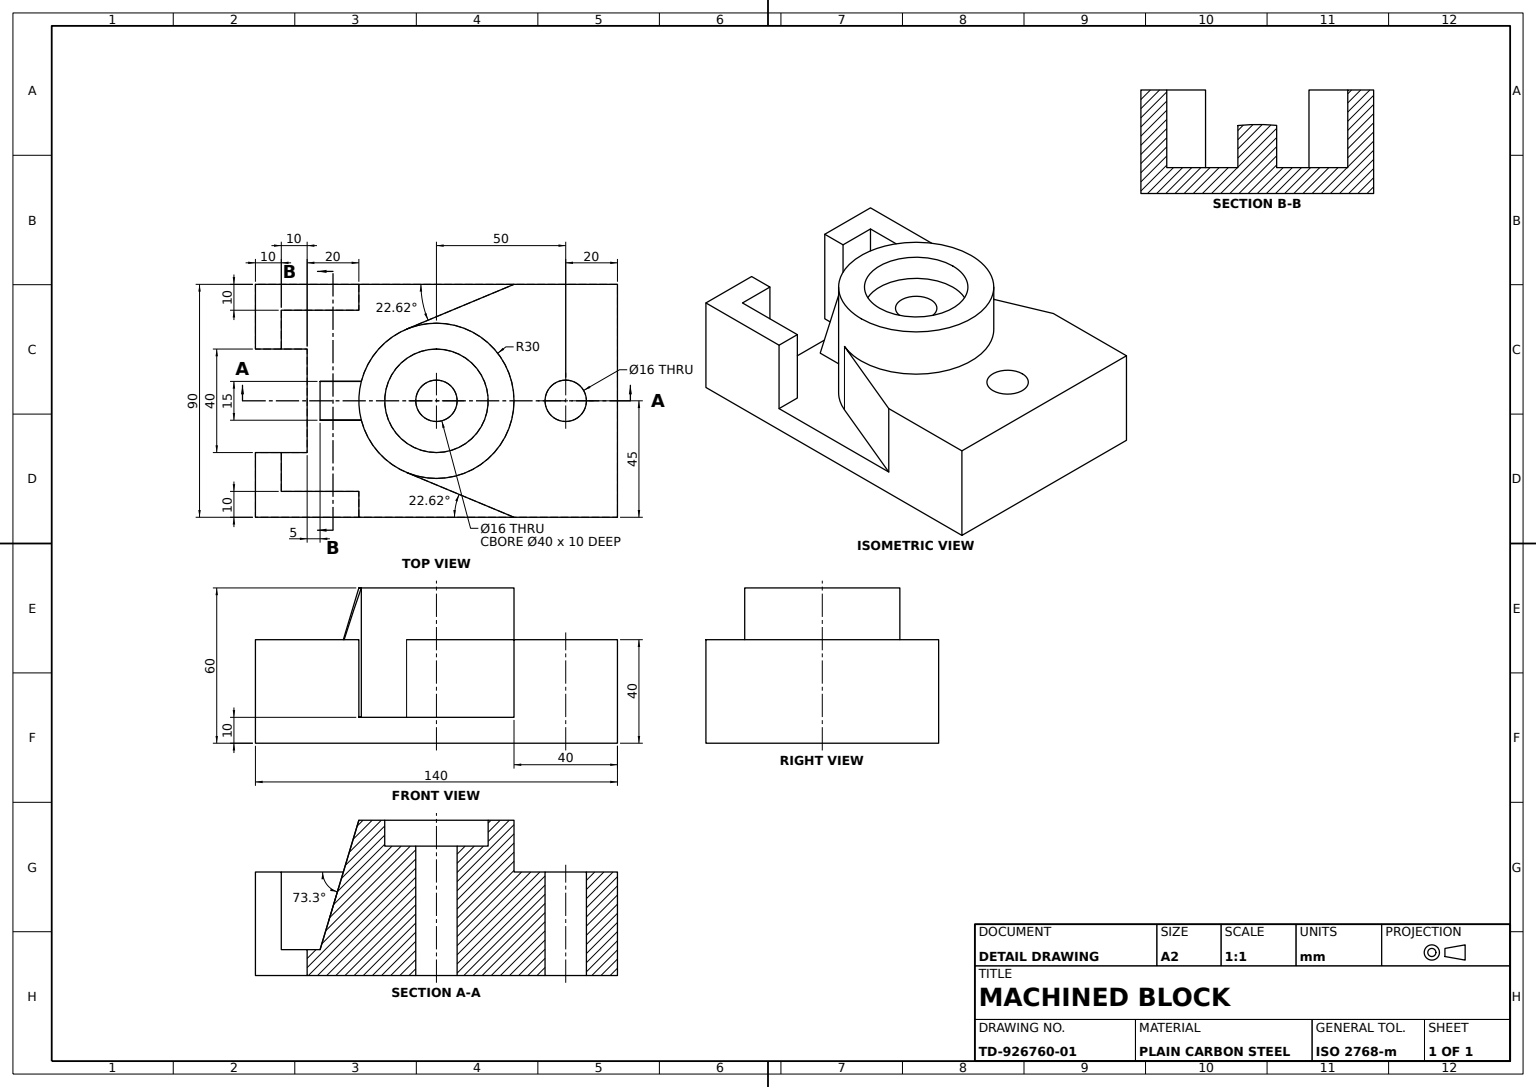
from build123d import *

# Parameters (mm, degrees)
BASE_PLATE_SKETCH_W        = 140
BASE_PLATE_SKETCH_H        = 90
BASE_PLATE_DEPTH           = 40
GLAND_BOSS_SKETCH_R        = 30
GLAND_BOSS_SKETCH_R_2      = 20
GLAND_BOSS_DEPTH           = 60
FORK_START                 = -30
FORK_CUTOUT_DEPTH          = 30
BORE_AND_HOLE_CUT_REACH    = 94.331
BORE_AND_HOLE_CUT_SKETCH_R = 8
BORE_AND_HOLE_CUT_SKETCH_W = 20
BORE_AND_HOLE_CUT_SKETCH_H = 40
SUPPORT_WEB_SKETCH_W       = 15.952624903
SUPPORT_WEB_SKETCH_H       = 15
SUPPORT_WEB_DEPTH          = 50
LIP_SKETCH_R               = 20
LIP_SKETCH_R_2             = 8
LIP_10MM_DEPTH             = 10


with BuildPart() as part:
    # Base Plate Sketch → Base Plate (new body)
    with BuildSketch(Plane(origin=(0, 0, 0), x_dir=(1, 0, 0), z_dir=(0, 1, 0))):
        Rectangle(BASE_PLATE_SKETCH_W, BASE_PLATE_SKETCH_H)
    extrude(amount=BASE_PLATE_DEPTH)

    # Gland Boss Sketch → Gland Boss (add)
    with BuildSketch(Plane(origin=(0, 0, 0), x_dir=(1, 0, 0), z_dir=(0, 1, 0))):
        with Locations(Location((0, 0, 0), (0, 0, 90))):
            Circle(GLAND_BOSS_SKETCH_R)
        with Locations(Location((0, 0, 0), (0, 0, 90))):
            Circle(GLAND_BOSS_SKETCH_R_2, mode=Mode.SUBTRACT)
    extrude(amount=GLAND_BOSS_DEPTH)

    # Fork Cutout Sketch → Fork Cutout (cut)
    with BuildSketch(Plane(origin=(0, 40, 0), x_dir=(1, 0, 0), z_dir=(0, 1, 0)).offset(FORK_START)):
        with BuildLine():
            Line((-70, 20), (-60, 20))
            Line((-60, 20), (-60, 35))
            Line((-60, 35), (-30, 35))
            Line((-30, 35), (-30, 45))
            Line((-30, 45), (30, 45))
            Line((30, 45), (-11.538461538, 27.692307692))
            ThreePointArc((-11.538461538, 27.692307692), (-30, 0), (-11.538461538, -27.692307692))
            Line((-11.538461538, -27.692307692), (30, -45))
            Line((30, -45), (-30, -45))
            Line((-30, -45), (-30, -35))
            Line((-30, -35), (-60, -35))
            Line((-60, -35), (-60, -20))
            Line((-60, -20), (-70, -20))
            Line((-70, -20), (-70, 20))
        make_face()
    extrude(amount=FORK_CUTOUT_DEPTH, mode=Mode.SUBTRACT)

    # Bore and Hole Cut Sketch → Bore and Hole Cut (cut, up to next)
    with BuildSketch(Plane(origin=(0, 40, 0), x_dir=(1, 0, 0), z_dir=(0, 1, 0)), mode=Mode.PRIVATE) as bore_and_hole_cut_sk1:
        with Locations(Location((0, 0, 0), (0, 0, 270))):
            Circle(BORE_AND_HOLE_CUT_SKETCH_R)
    bore_and_hole_cut_tool1 = extrude(bore_and_hole_cut_sk1.sketch, amount=-BORE_AND_HOLE_CUT_REACH, mode=Mode.PRIVATE) & part.part
    # Bore and Hole Cut Sketch → Bore and Hole Cut (cut, up to next)
    with BuildSketch(Plane(origin=(0, 40, 0), x_dir=(1, 0, 0), z_dir=(0, 1, 0)), mode=Mode.PRIVATE) as bore_and_hole_cut_sk2:
        with Locations(Location((50, 0, 0), (0, 0, 270))):
            Circle(BORE_AND_HOLE_CUT_SKETCH_R)
    bore_and_hole_cut_tool2 = extrude(bore_and_hole_cut_sk2.sketch, amount=-BORE_AND_HOLE_CUT_REACH, mode=Mode.PRIVATE) & part.part
    # Bore and Hole Cut Sketch → Bore and Hole Cut (cut, up to next)
    with BuildSketch(Plane(origin=(0, 40, 0), x_dir=(1, 0, 0), z_dir=(0, 1, 0)), mode=Mode.PRIVATE) as bore_and_hole_cut_sk3:
        with Locations((-60, 0)):
            Rectangle(BORE_AND_HOLE_CUT_SKETCH_W, BORE_AND_HOLE_CUT_SKETCH_H)
    bore_and_hole_cut_tool3 = extrude(bore_and_hole_cut_sk3.sketch, amount=-BORE_AND_HOLE_CUT_REACH, mode=Mode.PRIVATE) & part.part
    add(bore_and_hole_cut_tool1.solids().sort_by_distance((0, 40, 0))[0], mode=Mode.SUBTRACT)
    add(bore_and_hole_cut_tool2.solids().sort_by_distance((50, 40, 0))[0], mode=Mode.SUBTRACT)
    add(bore_and_hole_cut_tool3.solids().sort_by_distance((-60, 40, 0))[0], mode=Mode.SUBTRACT)

    # Support Web Sketch → Support Web (add)
    with BuildSketch(Plane(origin=(0, 60, 0), x_dir=(1, 0, 0), z_dir=(0, 1, 0))):
        with Locations((-37.023687548, 0)):
            Rectangle(SUPPORT_WEB_SKETCH_W, SUPPORT_WEB_SKETCH_H)
    extrude(amount=-SUPPORT_WEB_DEPTH)

    # Tapered Cut Start Profil for Tapered Lof → Tapered Lofted Cut section 0
    with BuildSketch(Plane(origin=(0, 60, 0), x_dir=(1, 0, 0), z_dir=(0, 1, 0))):
        with BuildLine():
            Line((-29.047375097, 7.5), (-45, 7.5))
            Line((-45, 7.5), (-45, -7.5))
            Line((-45, -7.5), (-29.047375097, -7.5))
            # circular arc as an exact rational Bezier (weights 1, cos(half-angle), 1)
            Bezier((-29.047375097, -7.5), (-30.98386677, 0), (-29.047375097, 7.5), weights=[1, 0.968245837, 1])
        make_face()
    # Tapered Cut End Profile → Tapered Lofted Cut section 1
    with BuildSketch(Plane(origin=(0, 10, 0), x_dir=(1, 0, 0), z_dir=(0, 1, 0))):
        with BuildLine():
            Line((-50, 15.482090991), (-45, 15.482090991))
            Line((-45, 15.482090991), (-45, -14.57582225))
            Line((-45, -14.57582225), (-50, -14.57582225))
            Line((-50, -14.57582225), (-50, 15.482090991))
        make_face()
    loft(mode=Mode.SUBTRACT)

    # Lip Sketch → Lip 10mm (add)
    with BuildSketch(Plane(origin=(0, 40, 0), x_dir=(1, 0, 0), z_dir=(0, 1, 0))):
        with Locations(Location((0, 0, 0), (0, 0, 270))):
            Circle(LIP_SKETCH_R)
        with Locations(Location((0, 0, 0), (0, 0, 270))):
            Circle(LIP_SKETCH_R_2, mode=Mode.SUBTRACT)
    extrude(amount=LIP_10MM_DEPTH)


solid = part.part
